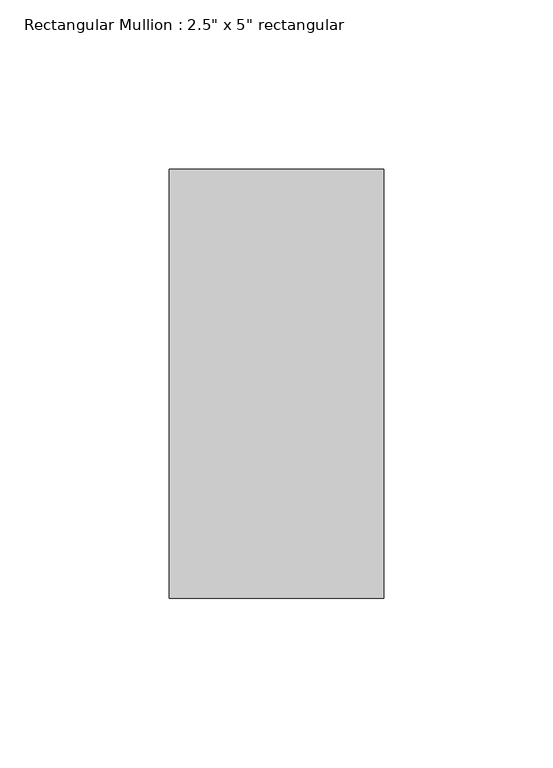
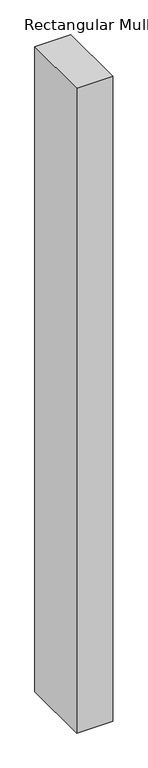
"""IFC4 building model written with IfcOpenShell, lengths in millimetres: member geometry."""

from ifc_helpers import new_model, si_unit, frame, origin, place, context, project, spatial, polyline, outline, extrude, source, transform, mapped, element, save


def member_e9c7f4a4(model_context):
    return source(origin(), model_context, "Body", "SweptSolid", [
        extrude(outline(polyline([(0.0, 63.5), (0.0, -63.5), (-63.5, -63.5), (-63.5, 63.5), (0.0, 63.5)])), frame((0.0, 0.0, -1200.15), z_axis=(0.0, 0.0, 1.0), x_axis=(1.0, 0.0, 0.0)), (0.0, 0.0, 1.0), 1200.15),
    ])


if __name__ == "__main__":
    model = new_model("IFC4")
    model_context = context("Model", 3, world=origin())
    ifc_project = project(units=[si_unit("LENGTHUNIT", "METRE", prefix="MILLI")], contexts=[model_context])
    site = spatial("IfcSite", under=ifc_project)
    building = spatial("IfcBuilding", under=site)
    placement = place(None, origin())
    member_shape = member_e9c7f4a4(model_context)
    element("IfcMember", 1, ObjectType="Rectangular Mullion : 2.5\" x 5\" rectangular", at=placement, inside=building, context=model_context, shape_type="MappedRepresentation", body=[
        mapped(member_shape, transform((0.0, 0.0, 0.0), x_axis=(1.0, 0.0, 0.0), y_axis=(0.0, 1.0, 0.0), z_axis=(0.0, 0.0, 1.0))),
    ])
    save(model, "model.ifc")

# Revit data of these elements
# Type "Rectangular Mullion : 2.5\" x 5\" rectangular"
#   built-in parameter 1007304 = 0.416667 (stored number, unit not read)
#   built-in parameter 1007301 = 0.104167 (stored number, unit not read)
#   built-in parameter 1007300 = 0.104167 (stored number, unit not read)
# Element 1 (IfcMember, "Rectangular Mullion : 2.5\" x 5\" rectangular")
#   Materials on its faces: "Rectangle 1 sq"
# Materials
#   "Rectangle 1 sq": class "Generic", colour RGB 120 120 120, transparency 0, Cost = 0
